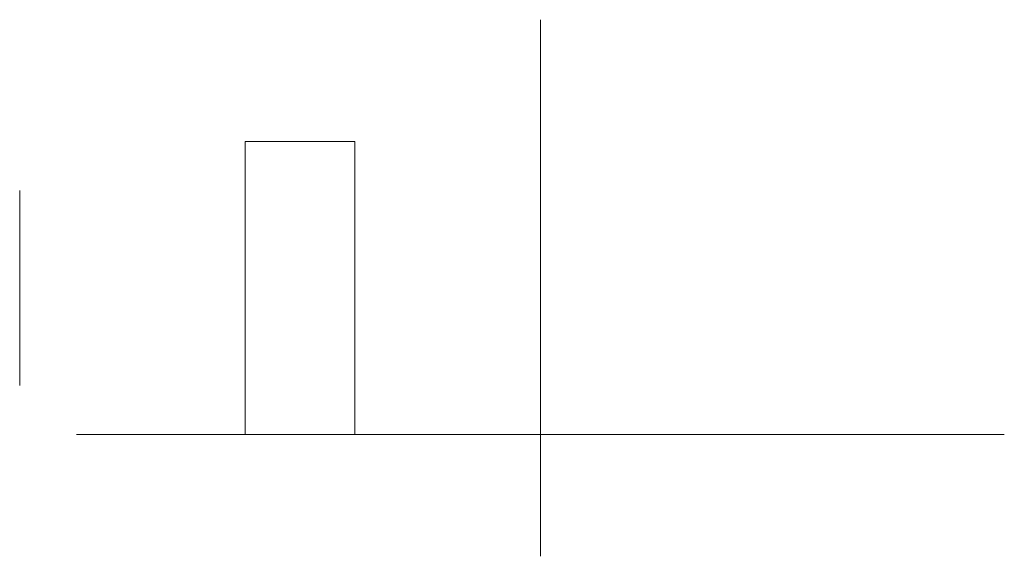
# Model space of a CAD drawing. Units: millimetres. Extents: x -87 to 690, y 0 to 52.
# Tile 1 of 1: x 608.96 to 689.62, y 8 to 52. Entities that reach past the tile are written whole.
import ezdxf

# ---------------------------------------------------------------- set-up
doc = ezdxf.new("R2010")
doc.units = ezdxf.units.MM
doc.layers.add('M-CONS', color=8, linetype='Continuous', lineweight=18)

msp = doc.modelspace()

# ---------------------------------------------------------------- linework, layer by layer
at = {"layer": 'M-CONS', "extrusion": (0, -1, 0)}
msp.add_line((651.624, 8, 3.519), (651.624, 52, 3.519), dxfattribs=at)
at = {"layer": 'M-CONS', "elevation": -3.481}
msp.add_lwpolyline([(636.426, 18), (627.426, 18), (627.426, 42), (636.426, 42)], close=True, dxfattribs=at)
at = {"layer": 'M-CONS', "extrusion": (-1, 0, 0), "elevation": -608.961}
msp.add_lwpolyline([(-22, -22.136), (-22, -58.136), (-38, -58.136), (-38, -22.136)], close=True, dxfattribs=at)
at = {"layer": 'M-CONS', "extrusion": (0, -1, 0), "elevation": -18}
msp.add_lwpolyline([(666.823, -3.481), (675.823, -3.481), (689.624, -41.481), (613.624, -41.481), (627.426, -3.481), (636.426, -3.481, -0.460566)], format="xyb", close=True, dxfattribs=at)
at = {"layer": 'M-CONS', "extrusion": (0, -1, 0)}
for radius in [20, 9]:
    msp.add_circle((651.624, -16.481, -18), radius, dxfattribs=at)

doc.saveas('drawing.dxf')
